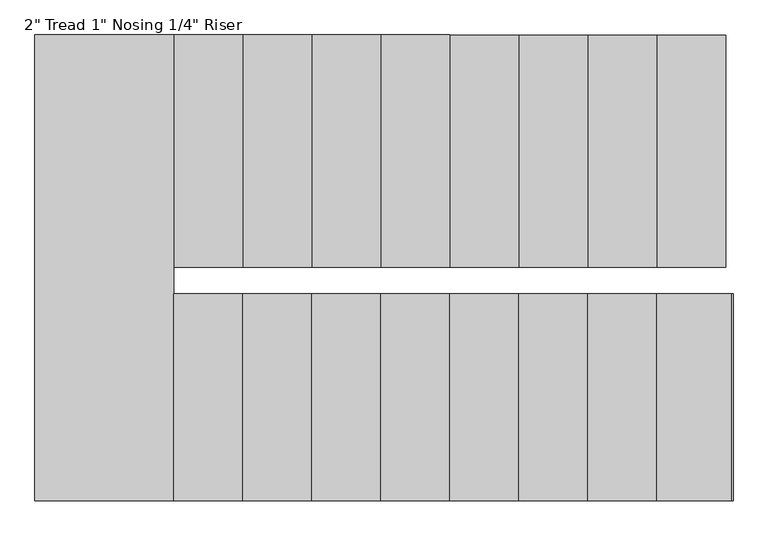
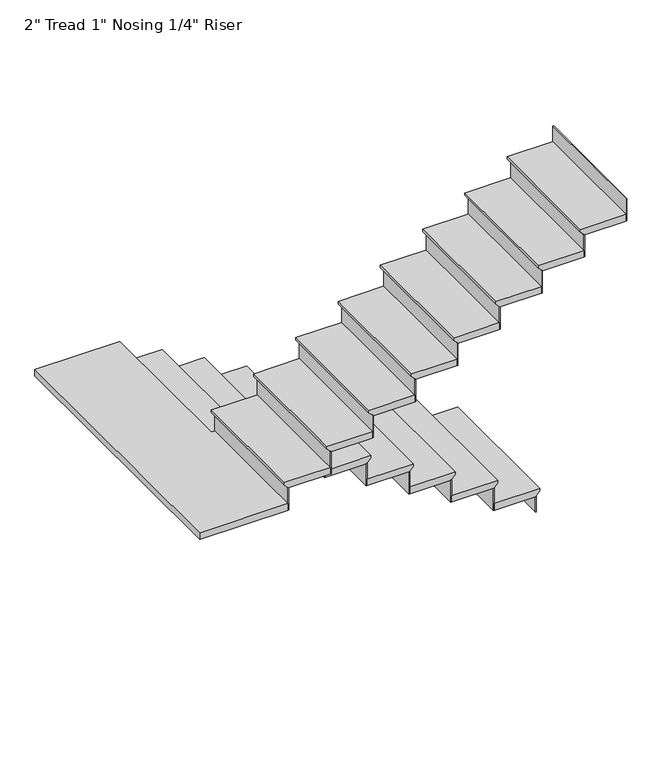
"""IFC4 building model written with IfcOpenShell, lengths in millimetres: stair flight geometry."""

from ifc_helpers import new_model, si_unit, origin, place, context, project, spatial, faceted_brep, source, transform, mapped, element, save


def stair_flight_3672e095(model_context):
    return source(origin(), model_context, "Body", "Brep", [
        faceted_brep([(4295.1355783, 9969.5, 9294.2833333), (4295.1355783, 9969.5, 9313.3333333), (4295.1355783, 8944.6068332, 9313.3333333), (4295.1355783, 8944.6068332, 9294.2833333), (4269.7355783, 9969.5, 9268.8833333), (4269.7355783, 8944.6068332, 9268.8833333), (3964.9355783, 9969.5, 9313.3333333), (3964.9355783, 8944.6068332, 9313.3333333), (4269.7355783, 8944.6068332, 9262.5333333), (3964.9355783, 8944.6068332, 9262.5333333), (3964.9355783, 9969.5, 9262.5333333), (4269.7355783, 9969.5, 9262.5333333)], [[[0, 1, 2, 3]], [[4, 0, 3, 5]], [[2, 1, 6, 7]], [[8, 9, 10, 11]], [[2, 7, 9, 8, 5, 3]], [[8, 11, 4, 5]], [[6, 1, 0, 4, 11, 10]], [[7, 6, 10, 9]]]),
        faceted_brep([(4269.7355783, 9969.5, 9262.5333333), (4269.7355783, 9969.5, 9144.0), (4263.3855783, 9969.5, 9144.0), (4263.3855783, 9969.5, 9262.5333333), (4269.7355783, 8944.6068332, 9262.5333333), (4263.3855783, 8944.6068332, 9262.5333333), (4263.3855783, 8944.6068332, 9144.0), (4269.7355783, 8944.6068332, 9144.0)], [[[0, 1, 2, 3]], [[4, 5, 6, 7]], [[1, 0, 4, 7]], [[2, 1, 7, 6]], [[3, 2, 6, 5]], [[0, 3, 5, 4]]]),
        faceted_brep([(3964.9355783, 9969.5, 9431.8666667), (3964.9355783, 9969.5, 9262.5333333), (3958.5855783, 9969.5, 9262.5333333), (3958.5855783, 9969.5, 9431.8666667), (3964.9355783, 8944.6068332, 9431.8666667), (3958.5855783, 8944.6068332, 9431.8666667), (3958.5855783, 8944.6068332, 9262.5333333), (3964.9355783, 8944.6068332, 9262.5333333)], [[[0, 1, 2, 3]], [[4, 5, 6, 7]], [[1, 0, 4, 7]], [[2, 1, 7, 6]], [[3, 2, 6, 5]], [[0, 3, 5, 4]]]),
        faceted_brep([(3990.3355783, 8944.6068332, 9482.6666667), (3990.3355783, 9969.5, 9482.6666667), (3660.1355783, 9969.5, 9482.6666667), (3660.1355783, 8944.6068332, 9482.6666667), (3964.9355783, 8944.6068332, 9431.8666667), (3660.1355783, 8944.6068332, 9431.8666667), (3660.1355783, 9969.5, 9431.8666667), (3964.9355783, 9969.5, 9431.8666667), (3964.9355783, 8944.6068332, 9438.2166667), (3990.3355783, 8944.6068332, 9463.6166667), (3964.9355783, 9969.5, 9438.2166667), (3990.3355783, 9969.5, 9463.6166667)], [[[0, 1, 2, 3]], [[4, 5, 6, 7]], [[0, 3, 5, 4, 8, 9]], [[4, 7, 10, 8]], [[2, 1, 11, 10, 7, 6]], [[3, 2, 6, 5]], [[11, 1, 0, 9]], [[10, 11, 9, 8]]]),
        faceted_brep([(3660.1355783, 9969.5, 9601.2), (3660.1355783, 9969.5, 9431.8666667), (3653.7855783, 9969.5, 9431.8666667), (3653.7855783, 9969.5, 9601.2), (3660.1355783, 8944.6068332, 9601.2), (3653.7855783, 8944.6068332, 9601.2), (3653.7855783, 8944.6068332, 9431.8666667), (3660.1355783, 8944.6068332, 9431.8666667)], [[[0, 1, 2, 3]], [[4, 5, 6, 7]], [[1, 0, 4, 7]], [[2, 1, 7, 6]], [[3, 2, 6, 5]], [[0, 3, 5, 4]]]),
        faceted_brep([(3685.5355783, 8944.6068332, 9652.0), (3685.5355783, 9969.5, 9652.0), (3355.3355783, 9969.5, 9652.0), (3355.3355783, 8944.6068332, 9652.0), (3660.1355783, 8944.6068332, 9601.2), (3355.3355783, 8944.6068332, 9601.2), (3355.3355783, 9969.5, 9601.2), (3660.1355783, 9969.5, 9601.2), (3660.1355783, 8944.6068332, 9607.55), (3685.5355783, 8944.6068332, 9632.95), (3660.1355783, 9969.5, 9607.55), (3685.5355783, 9969.5, 9632.95)], [[[0, 1, 2, 3]], [[4, 5, 6, 7]], [[0, 3, 5, 4, 8, 9]], [[4, 7, 10, 8]], [[2, 1, 11, 10, 7, 6]], [[3, 2, 6, 5]], [[11, 1, 0, 9]], [[10, 11, 9, 8]]]),
        faceted_brep([(3355.3355783, 9969.5, 9770.5333333), (3355.3355783, 9969.5, 9601.2), (3348.9855783, 9969.5, 9601.2), (3348.9855783, 9969.5, 9770.5333333), (3355.3355783, 8944.6068332, 9770.5333333), (3348.9855783, 8944.6068332, 9770.5333333), (3348.9855783, 8944.6068332, 9601.2), (3355.3355783, 8944.6068332, 9601.2)], [[[0, 1, 2, 3]], [[4, 5, 6, 7]], [[1, 0, 4, 7]], [[2, 1, 7, 6]], [[3, 2, 6, 5]], [[0, 3, 5, 4]]]),
        faceted_brep([(3380.7355783, 8944.6068332, 9821.3333333), (3380.7355783, 9969.5, 9821.3333333), (3050.5355783, 9969.5, 9821.3333333), (3050.5355783, 8944.6068332, 9821.3333333), (3355.3355783, 8944.6068332, 9770.5333333), (3050.5355783, 8944.6068332, 9770.5333333), (3050.5355783, 9969.5, 9770.5333333), (3355.3355783, 9969.5, 9770.5333333), (3355.3355783, 8944.6068332, 9776.8833333), (3380.7355783, 8944.6068332, 9802.2833333), (3355.3355783, 9969.5, 9776.8833333), (3380.7355783, 9969.5, 9802.2833333)], [[[0, 1, 2, 3]], [[4, 5, 6, 7]], [[0, 3, 5, 4, 8, 9]], [[4, 7, 10, 8]], [[2, 1, 11, 10, 7, 6]], [[3, 2, 6, 5]], [[11, 1, 0, 9]], [[10, 11, 9, 8]]]),
        faceted_brep([(3050.5355783, 9969.5, 9939.8666667), (3050.5355783, 9969.5, 9770.5333333), (3044.1855783, 9969.5, 9770.5333333), (3044.1855783, 9969.5, 9939.8666667), (3050.5355783, 8944.6068332, 9939.8666667), (3044.1855783, 8944.6068332, 9939.8666667), (3044.1855783, 8944.6068332, 9770.5333333), (3050.5355783, 8944.6068332, 9770.5333333)], [[[0, 1, 2, 3]], [[4, 5, 6, 7]], [[1, 0, 4, 7]], [[2, 1, 7, 6]], [[3, 2, 6, 5]], [[0, 3, 5, 4]]]),
        faceted_brep([(3075.9355783, 8944.6068332, 9990.6666667), (3075.9355783, 9969.5, 9990.6666667), (2745.7355783, 9969.5, 9990.6666667), (2745.7355783, 8944.6068332, 9990.6666667), (3050.5355783, 8944.6068332, 9939.8666667), (2745.7355783, 8944.6068332, 9939.8666667), (2745.7355783, 9969.5, 9939.8666667), (3050.5355783, 9969.5, 9939.8666667), (3050.5355783, 8944.6068332, 9946.2166667), (3075.9355783, 8944.6068332, 9971.6166667), (3050.5355783, 9969.5, 9946.2166667), (3075.9355783, 9969.5, 9971.6166667)], [[[0, 1, 2, 3]], [[4, 5, 6, 7]], [[0, 3, 5, 4, 8, 9]], [[4, 7, 10, 8]], [[2, 1, 11, 10, 7, 6]], [[3, 2, 6, 5]], [[11, 1, 0, 9]], [[10, 11, 9, 8]]]),
        faceted_brep([(2745.7355783, 9969.5, 10109.2), (2745.7355783, 9969.5, 9939.8666667), (2739.3855783, 9969.5, 9939.8666667), (2739.3855783, 9969.5, 10109.2), (2745.7355783, 8944.6068332, 10109.2), (2739.3855783, 8944.6068332, 10109.2), (2739.3855783, 8944.6068332, 9939.8666667), (2745.7355783, 8944.6068332, 9939.8666667)], [[[0, 1, 2, 3]], [[4, 5, 6, 7]], [[1, 0, 4, 7]], [[2, 1, 7, 6]], [[3, 2, 6, 5]], [[0, 3, 5, 4]]]),
        faceted_brep([(2771.1355783, 8944.6068332, 10160.0), (2771.1355783, 9969.5, 10160.0), (2440.9355783, 9969.5, 10160.0), (2440.9355783, 8944.6068332, 10160.0), (2745.7355783, 8944.6068332, 10109.2), (2440.9355783, 8944.6068332, 10109.2), (2440.9355783, 9969.5, 10109.2), (2745.7355783, 9969.5, 10109.2), (2745.7355783, 8944.6068332, 10115.55), (2771.1355783, 8944.6068332, 10140.95), (2745.7355783, 9969.5, 10115.55), (2771.1355783, 9969.5, 10140.95)], [[[0, 1, 2, 3]], [[4, 5, 6, 7]], [[0, 3, 5, 4, 8, 9]], [[4, 7, 10, 8]], [[2, 1, 11, 10, 7, 6]], [[3, 2, 6, 5]], [[11, 1, 0, 9]], [[10, 11, 9, 8]]]),
        faceted_brep([(2440.9355783, 9969.5, 10278.5333333), (2440.9355783, 9969.5, 10109.2), (2434.5855783, 9969.5, 10109.2), (2434.5855783, 9969.5, 10278.5333333), (2440.9355783, 8944.6068332, 10278.5333333), (2434.5855783, 8944.6068332, 10278.5333333), (2434.5855783, 8944.6068332, 10109.2), (2440.9355783, 8944.6068332, 10109.2)], [[[0, 1, 2, 3]], [[4, 5, 6, 7]], [[1, 0, 4, 7]], [[2, 1, 7, 6]], [[3, 2, 6, 5]], [[0, 3, 5, 4]]]),
        faceted_brep([(2466.3355783, 8944.6068332, 10329.3333333), (2466.3355783, 9969.5, 10329.3333333), (2136.1355783, 9969.5, 10329.3333333), (2136.1355783, 8944.6068332, 10329.3333333), (2440.9355783, 8944.6068332, 10278.5333333), (2136.1355783, 8944.6068332, 10278.5333333), (2136.1355783, 9969.5, 10278.5333333), (2440.9355783, 9969.5, 10278.5333333), (2440.9355783, 8944.6068332, 10284.8833333), (2466.3355783, 8944.6068332, 10310.2833333), (2440.9355783, 9969.5, 10284.8833333), (2466.3355783, 9969.5, 10310.2833333)], [[[0, 1, 2, 3]], [[4, 5, 6, 7]], [[0, 3, 5, 4, 8, 9]], [[4, 7, 10, 8]], [[2, 1, 11, 10, 7, 6]], [[3, 2, 6, 5]], [[11, 1, 0, 9]], [[10, 11, 9, 8]]]),
        faceted_brep([(2136.1355783, 9969.5, 10447.8666667), (2136.1355783, 9969.5, 10278.5333333), (2129.7855783, 9969.5, 10278.5333333), (2129.7855783, 9969.5, 10447.8666667), (2136.1355783, 8944.6068332, 10447.8666667), (2129.7855783, 8944.6068332, 10447.8666667), (2129.7855783, 8944.6068332, 10278.5333333), (2136.1355783, 8944.6068332, 10278.5333333)], [[[0, 1, 2, 3]], [[4, 5, 6, 7]], [[1, 0, 4, 7]], [[2, 1, 7, 6]], [[3, 2, 6, 5]], [[0, 3, 5, 4]]]),
        faceted_brep([(2161.5355783, 8944.6068332, 10498.6666667), (2161.5355783, 9969.5, 10498.6666667), (1831.3355783, 9969.5, 10498.6666667), (1831.3355783, 8944.6068332, 10498.6666667), (2136.1355783, 8944.6068332, 10447.8666667), (1831.3355783, 8944.6068332, 10447.8666667), (1831.3355783, 9969.5, 10447.8666667), (2136.1355783, 9969.5, 10447.8666667), (2136.1355783, 8944.6068332, 10454.2166667), (2161.5355783, 8944.6068332, 10479.6166667), (2136.1355783, 9969.5, 10454.2166667), (2161.5355783, 9969.5, 10479.6166667)], [[[0, 1, 2, 3]], [[4, 5, 6, 7]], [[0, 3, 5, 4, 8, 9]], [[4, 7, 10, 8]], [[2, 1, 11, 10, 7, 6]], [[3, 2, 6, 5]], [[11, 1, 0, 9]], [[10, 11, 9, 8]]]),
        faceted_brep([(1831.3355783, 9969.5, 10617.2), (1831.3355783, 9969.5, 10447.8666667), (1824.9855783, 9969.5, 10447.8666667), (1824.9855783, 9969.5, 10617.2), (1831.3355783, 8944.6068332, 10617.2), (1824.9855783, 8944.6068332, 10617.2), (1824.9855783, 8944.6068332, 10447.8666667), (1831.3355783, 8944.6068332, 10447.8666667)], [[[0, 1, 2, 3]], [[4, 5, 6, 7]], [[1, 0, 4, 7]], [[2, 1, 7, 6]], [[3, 2, 6, 5]], [[0, 3, 5, 4]]]),
        faceted_brep([(1882.1355783, 8826.5, 10668.0), (1856.7355783, 8826.5, 10668.0), (1856.7355783, 9969.5, 10668.0), (1244.6, 9969.5, 10668.0), (1244.6, 7912.1, 10668.0), (1882.1355783, 7912.1, 10668.0), (1856.7355783, 8826.5, 10617.2), (1882.1355783, 8826.5, 10617.2), (1882.1355783, 7912.1, 10617.2), (1244.6, 7912.1, 10617.2), (1244.6, 9969.5, 10617.2), (1831.3355783, 9969.5, 10617.2), (1831.3355783, 8944.6068332, 10617.2), (1856.7355783, 8944.6068332, 10617.2), (1856.7355783, 8944.6068332, 10648.95), (1856.7355783, 9969.5, 10648.95), (1831.3355783, 8944.6068332, 10623.55), (1831.3355783, 9969.5, 10623.55)], [[[0, 1, 2, 3, 4, 5]], [[6, 7, 8, 9, 10, 11, 12, 13]], [[1, 0, 7, 6]], [[2, 1, 6, 13, 14, 15]], [[13, 12, 16, 14]], [[12, 11, 17, 16]], [[3, 2, 15, 17, 11, 10]], [[4, 3, 10, 9]], [[5, 4, 9, 8]], [[0, 5, 8, 7]], [[17, 15, 14, 16]]]),
        faceted_brep([(1882.1355783, 7912.1, 10786.5333333), (1882.1355783, 7912.1, 10617.2), (1888.4855783, 7912.1, 10617.2), (1888.4855783, 7912.1, 10786.5333333), (1882.1355783, 8826.5, 10786.5333333), (1888.4855783, 8826.5, 10786.5333333), (1888.4855783, 8826.5, 10617.2), (1882.1355783, 8826.5, 10617.2)], [[[0, 1, 2, 3]], [[4, 5, 6, 7]], [[1, 0, 4, 7]], [[2, 1, 7, 6]], [[3, 2, 6, 5]], [[0, 3, 5, 4]]]),
        faceted_brep([(1856.7355783, 8826.5, 10837.3333333), (1856.7355783, 7912.1, 10837.3333333), (2186.9355783, 7912.1, 10837.3333333), (2186.9355783, 8826.5, 10837.3333333), (1882.1355783, 8826.5, 10786.5333333), (2186.9355783, 8826.5, 10786.5333333), (2186.9355783, 7912.1, 10786.5333333), (1882.1355783, 7912.1, 10786.5333333), (1882.1355783, 8826.5, 10792.8833333), (1856.7355783, 8826.5, 10818.2833333), (1882.1355783, 7912.1, 10792.8833333), (1856.7355783, 7912.1, 10818.2833333)], [[[0, 1, 2, 3]], [[4, 5, 6, 7]], [[0, 3, 5, 4, 8, 9]], [[4, 7, 10, 8]], [[2, 1, 11, 10, 7, 6]], [[3, 2, 6, 5]], [[11, 1, 0, 9]], [[10, 11, 9, 8]]]),
        faceted_brep([(2186.9355783, 7912.1, 10955.8666667), (2186.9355783, 7912.1, 10786.5333333), (2193.2855783, 7912.1, 10786.5333333), (2193.2855783, 7912.1, 10955.8666667), (2186.9355783, 8826.5, 10955.8666667), (2193.2855783, 8826.5, 10955.8666667), (2193.2855783, 8826.5, 10786.5333333), (2186.9355783, 8826.5, 10786.5333333)], [[[0, 1, 2, 3]], [[4, 5, 6, 7]], [[1, 0, 4, 7]], [[2, 1, 7, 6]], [[3, 2, 6, 5]], [[0, 3, 5, 4]]]),
        faceted_brep([(2161.5355783, 8826.5, 11006.6666667), (2161.5355783, 7912.1, 11006.6666667), (2491.7355783, 7912.1, 11006.6666667), (2491.7355783, 8826.5, 11006.6666667), (2186.9355783, 8826.5, 10955.8666667), (2491.7355783, 8826.5, 10955.8666667), (2491.7355783, 7912.1, 10955.8666667), (2186.9355783, 7912.1, 10955.8666667), (2186.9355783, 8826.5, 10962.2166667), (2161.5355783, 8826.5, 10987.6166667), (2186.9355783, 7912.1, 10962.2166667), (2161.5355783, 7912.1, 10987.6166667)], [[[0, 1, 2, 3]], [[4, 5, 6, 7]], [[0, 3, 5, 4, 8, 9]], [[4, 7, 10, 8]], [[2, 1, 11, 10, 7, 6]], [[3, 2, 6, 5]], [[11, 1, 0, 9]], [[10, 11, 9, 8]]]),
        faceted_brep([(2491.7355783, 7912.1, 11125.2), (2491.7355783, 7912.1, 10955.8666667), (2498.0855783, 7912.1, 10955.8666667), (2498.0855783, 7912.1, 11125.2), (2491.7355783, 8826.5, 11125.2), (2498.0855783, 8826.5, 11125.2), (2498.0855783, 8826.5, 10955.8666667), (2491.7355783, 8826.5, 10955.8666667)], [[[0, 1, 2, 3]], [[4, 5, 6, 7]], [[1, 0, 4, 7]], [[2, 1, 7, 6]], [[3, 2, 6, 5]], [[0, 3, 5, 4]]]),
        faceted_brep([(2466.3355783, 8826.5, 11176.0), (2466.3355783, 7912.1, 11176.0), (2796.5355783, 7912.1, 11176.0), (2796.5355783, 8826.5, 11176.0), (2491.7355783, 8826.5, 11125.2), (2796.5355783, 8826.5, 11125.2), (2796.5355783, 7912.1, 11125.2), (2491.7355783, 7912.1, 11125.2), (2491.7355783, 8826.5, 11131.55), (2466.3355783, 8826.5, 11156.95), (2491.7355783, 7912.1, 11131.55), (2466.3355783, 7912.1, 11156.95)], [[[0, 1, 2, 3]], [[4, 5, 6, 7]], [[0, 3, 5, 4, 8, 9]], [[4, 7, 10, 8]], [[2, 1, 11, 10, 7, 6]], [[3, 2, 6, 5]], [[11, 1, 0, 9]], [[10, 11, 9, 8]]]),
        faceted_brep([(2796.5355783, 7912.1, 11294.5333333), (2796.5355783, 7912.1, 11125.2), (2802.8855783, 7912.1, 11125.2), (2802.8855783, 7912.1, 11294.5333333), (2796.5355783, 8826.5, 11294.5333333), (2802.8855783, 8826.5, 11294.5333333), (2802.8855783, 8826.5, 11125.2), (2796.5355783, 8826.5, 11125.2)], [[[0, 1, 2, 3]], [[4, 5, 6, 7]], [[1, 0, 4, 7]], [[2, 1, 7, 6]], [[3, 2, 6, 5]], [[0, 3, 5, 4]]]),
        faceted_brep([(2771.1355783, 8826.5, 11345.3333333), (2771.1355783, 7912.1, 11345.3333333), (3101.3355783, 7912.1, 11345.3333333), (3101.3355783, 8826.5, 11345.3333333), (2796.5355783, 8826.5, 11294.5333333), (3101.3355783, 8826.5, 11294.5333333), (3101.3355783, 7912.1, 11294.5333333), (2796.5355783, 7912.1, 11294.5333333), (2796.5355783, 8826.5, 11300.8833333), (2771.1355783, 8826.5, 11326.2833333), (2796.5355783, 7912.1, 11300.8833333), (2771.1355783, 7912.1, 11326.2833333)], [[[0, 1, 2, 3]], [[4, 5, 6, 7]], [[0, 3, 5, 4, 8, 9]], [[4, 7, 10, 8]], [[2, 1, 11, 10, 7, 6]], [[3, 2, 6, 5]], [[11, 1, 0, 9]], [[10, 11, 9, 8]]]),
        faceted_brep([(3101.3355783, 7912.1, 11463.8666667), (3101.3355783, 7912.1, 11294.5333333), (3107.6855783, 7912.1, 11294.5333333), (3107.6855783, 7912.1, 11463.8666667), (3101.3355783, 8826.5, 11463.8666667), (3107.6855783, 8826.5, 11463.8666667), (3107.6855783, 8826.5, 11294.5333333), (3101.3355783, 8826.5, 11294.5333333)], [[[0, 1, 2, 3]], [[4, 5, 6, 7]], [[1, 0, 4, 7]], [[2, 1, 7, 6]], [[3, 2, 6, 5]], [[0, 3, 5, 4]]]),
        faceted_brep([(3075.9355783, 8826.5, 11514.6666667), (3075.9355783, 7912.1, 11514.6666667), (3406.1355783, 7912.1, 11514.6666667), (3406.1355783, 8826.5, 11514.6666667), (3101.3355783, 8826.5, 11463.8666667), (3406.1355783, 8826.5, 11463.8666667), (3406.1355783, 7912.1, 11463.8666667), (3101.3355783, 7912.1, 11463.8666667), (3101.3355783, 8826.5, 11470.2166667), (3075.9355783, 8826.5, 11495.6166667), (3101.3355783, 7912.1, 11470.2166667), (3075.9355783, 7912.1, 11495.6166667)], [[[0, 1, 2, 3]], [[4, 5, 6, 7]], [[0, 3, 5, 4, 8, 9]], [[4, 7, 10, 8]], [[2, 1, 11, 10, 7, 6]], [[3, 2, 6, 5]], [[11, 1, 0, 9]], [[10, 11, 9, 8]]]),
        faceted_brep([(3406.1355783, 7912.1, 11633.2), (3406.1355783, 7912.1, 11463.8666667), (3412.4855783, 7912.1, 11463.8666667), (3412.4855783, 7912.1, 11633.2), (3406.1355783, 8826.5, 11633.2), (3412.4855783, 8826.5, 11633.2), (3412.4855783, 8826.5, 11463.8666667), (3406.1355783, 8826.5, 11463.8666667)], [[[0, 1, 2, 3]], [[4, 5, 6, 7]], [[1, 0, 4, 7]], [[2, 1, 7, 6]], [[3, 2, 6, 5]], [[0, 3, 5, 4]]]),
        faceted_brep([(3380.7355783, 8826.5, 11684.0), (3380.7355783, 7912.1, 11684.0), (3710.9355783, 7912.1, 11684.0), (3710.9355783, 8826.5, 11684.0), (3406.1355783, 8826.5, 11633.2), (3710.9355783, 8826.5, 11633.2), (3710.9355783, 7912.1, 11633.2), (3406.1355783, 7912.1, 11633.2), (3406.1355783, 8826.5, 11639.55), (3380.7355783, 8826.5, 11664.95), (3406.1355783, 7912.1, 11639.55), (3380.7355783, 7912.1, 11664.95)], [[[0, 1, 2, 3]], [[4, 5, 6, 7]], [[0, 3, 5, 4, 8, 9]], [[4, 7, 10, 8]], [[2, 1, 11, 10, 7, 6]], [[3, 2, 6, 5]], [[11, 1, 0, 9]], [[10, 11, 9, 8]]]),
        faceted_brep([(3710.9355783, 7912.1, 11802.5333333), (3710.9355783, 7912.1, 11633.2), (3717.2855783, 7912.1, 11633.2), (3717.2855783, 7912.1, 11802.5333333), (3710.9355783, 8826.5, 11802.5333333), (3717.2855783, 8826.5, 11802.5333333), (3717.2855783, 8826.5, 11633.2), (3710.9355783, 8826.5, 11633.2)], [[[0, 1, 2, 3]], [[4, 5, 6, 7]], [[1, 0, 4, 7]], [[2, 1, 7, 6]], [[3, 2, 6, 5]], [[0, 3, 5, 4]]]),
        faceted_brep([(3685.5355783, 8826.5, 11853.3333333), (3685.5355783, 7912.1, 11853.3333333), (4015.7355783, 7912.1, 11853.3333333), (4015.7355783, 8826.5, 11853.3333333), (3710.9355783, 8826.5, 11802.5333333), (4015.7355783, 8826.5, 11802.5333333), (4015.7355783, 7912.1, 11802.5333333), (3710.9355783, 7912.1, 11802.5333333), (3710.9355783, 8826.5, 11808.8833333), (3685.5355783, 8826.5, 11834.2833333), (3710.9355783, 7912.1, 11808.8833333), (3685.5355783, 7912.1, 11834.2833333)], [[[0, 1, 2, 3]], [[4, 5, 6, 7]], [[0, 3, 5, 4, 8, 9]], [[4, 7, 10, 8]], [[2, 1, 11, 10, 7, 6]], [[3, 2, 6, 5]], [[11, 1, 0, 9]], [[10, 11, 9, 8]]]),
        faceted_brep([(4015.7355783, 7912.1, 11971.8666667), (4015.7355783, 7912.1, 11802.5333333), (4022.0855783, 7912.1, 11802.5333333), (4022.0855783, 7912.1, 11971.8666667), (4015.7355783, 8826.5, 11971.8666667), (4022.0855783, 8826.5, 11971.8666667), (4022.0855783, 8826.5, 11802.5333333), (4015.7355783, 8826.5, 11802.5333333)], [[[0, 1, 2, 3]], [[4, 5, 6, 7]], [[1, 0, 4, 7]], [[2, 1, 7, 6]], [[3, 2, 6, 5]], [[0, 3, 5, 4]]]),
        faceted_brep([(4320.5355783, 7912.1, 12141.2), (4320.5355783, 7912.1, 11971.8666667), (4326.8855783, 7912.1, 11971.8666667), (4326.8855783, 7912.1, 12141.2), (4320.5355783, 8826.5, 12141.2), (4326.8855783, 8826.5, 12141.2), (4326.8855783, 8826.5, 11971.8666667), (4320.5355783, 8826.5, 11971.8666667)], [[[0, 1, 2, 3]], [[4, 5, 6, 7]], [[1, 0, 4, 7]], [[2, 1, 7, 6]], [[3, 2, 6, 5]], [[0, 3, 5, 4]]]),
        faceted_brep([(3990.3355783, 8826.5, 12022.6666667), (3990.3355783, 7912.1, 12022.6666667), (4320.5355783, 7912.1, 12022.6666667), (4320.5355783, 8826.5, 12022.6666667), (4015.7355783, 8826.5, 11971.8666667), (4320.5355783, 8826.5, 11971.8666667), (4320.5355783, 7912.1, 11971.8666667), (4015.7355783, 7912.1, 11971.8666667), (4015.7355783, 8826.5, 11978.2166667), (3990.3355783, 8826.5, 12003.6166667), (4015.7355783, 7912.1, 11978.2166667), (3990.3355783, 7912.1, 12003.6166667)], [[[0, 1, 2, 3]], [[4, 5, 6, 7]], [[0, 3, 5, 4, 8, 9]], [[4, 7, 10, 8]], [[2, 1, 11, 10, 7, 6]], [[3, 2, 6, 5]], [[11, 1, 0, 9]], [[10, 11, 9, 8]]]),
    ])


if __name__ == "__main__":
    model = new_model("IFC4")
    model_context = context("Model", 3, world=origin())
    ifc_project = project(units=[si_unit("LENGTHUNIT", "METRE", prefix="MILLI")], contexts=[model_context])
    site = spatial("IfcSite", under=ifc_project)
    building = spatial("IfcBuilding", under=site)
    placement = place(None, origin())
    stair_flight_shape = stair_flight_3672e095(model_context)
    element("IfcStairFlight", 1, ObjectType="2\" Tread 1\" Nosing 1/4\" Riser", at=placement, inside=building, context=model_context, shape_type="MappedRepresentation", body=[
        mapped(stair_flight_shape, transform((0.0, 0.0, 0.0), x_axis=(1.0, 0.0, 0.0), y_axis=(0.0, 1.0, 0.0), z_axis=(0.0, 0.0, 1.0))),
    ])
    save(model, "model.ifc")
